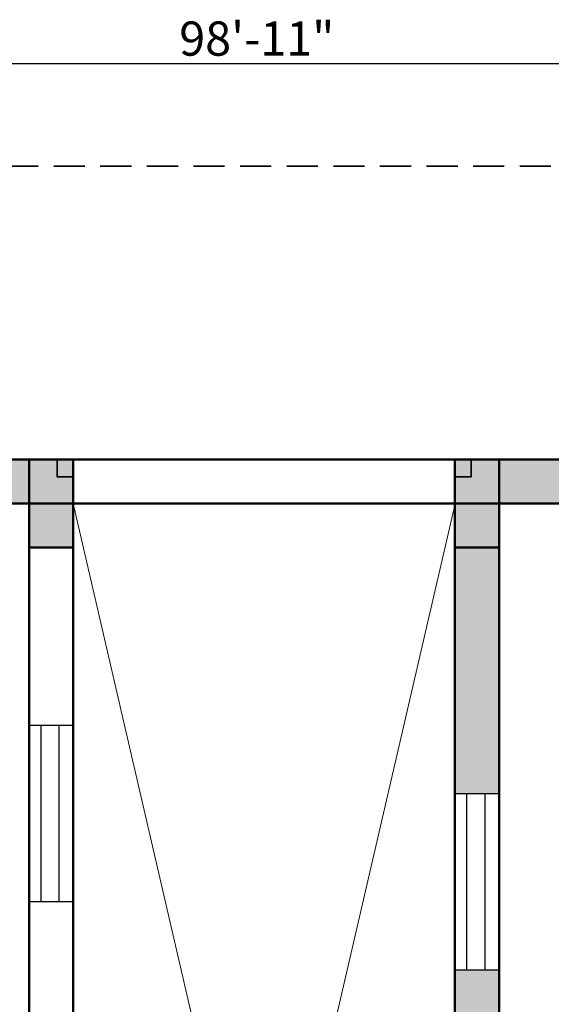
# Model space of a CAD drawing. Units: inches. Extents: x -7 to 1228, y -146 to 1091.
# Tile 77 of 88: x 545 to 654, y 890 to 1091. Entities that reach past the tile are written whole.
import ezdxf

# ---------------------------------------------------------------- set-up
doc = ezdxf.new("R2010")
doc.units = ezdxf.units.IN
doc.linetypes.add('DASHED2', pattern=[9.525, 6.35, -3.175])
for name, color, linetype, lineweight in [('A-ANNO-DIMS', 2, 'Continuous', 18), ('A-COLS', 6, 'Continuous', 35), ('A-FLOR-VOID', 7, 'Continuous', 18), ('A-GLAZ', 175, 'Continuous', 25), ('A-WALL', 7, 'Continuous', 50), ('A-WALL-PATT', 251, 'Continuous', 13), ('C-PROP', 1, 'DASHED2', 35)]:
    doc.layers.add(name, color=color, linetype=linetype, lineweight=lineweight)
doc.styles.get("Standard").update_dxf_attribs({"font": 'arial.ttf'})
doc.dimstyles.new('ISO-25', dxfattribs={"dimtxt": 7, "dimasz": 4, "dimexe": 1.25, "dimexo": 0.625, "dimtad": 1, "dimdec": 1, "dimlunit": 3, "dimtxsty": 'Standard', "dimcen": 2.5, "dimadec": 0, "dimazin": 0, "dimtfac": 1, "dimtdec": 1, "dimtmove": 1, "dimatfit": 3, "dimfxl": 1, "dimarcsym": 0})

# ---------------------------------------------------------------- blocks, each defined once
blk = doc.blocks.new('*D11')
at = {"layer": 'A-ANNO-DIMS', "color": 0, "lineweight": -2, "transparency": 16777216}
for p, q in [((0, 1061.62), (0, 1083.25)), ((4, 1082), (1183, 1082)), ((1187, 1061.62), (1187, 1083.25))]:
    blk.add_line(p, q, dxfattribs=at)
at = {"layer": 'A-ANNO-DIMS', "color": 0, "transparency": 16777216}
for points in [[(4, 1082.67), (4, 1081.33), (0, 1082)], [(1183, 1082.67), (1183, 1081.33), (1187, 1082)]]:
    blk.add_solid(points, dxfattribs=at)
at = {"layer": 'Defpoints', "color": 0, "transparency": 16777216}
for p in [(1187, 1082), (0, 1061), (1187, 1061)]:
    blk.add_point(p, dxfattribs=at)
at = {"layer": 'A-ANNO-DIMS', "color": 0, "transparency": 16777216, "insert": (593.5, 1086.2), "char_height": 7, "attachment_point": 5}
blk.add_mtext('98\'-11"', dxfattribs=at)
blk = doc.blocks.new('WIN-36')
for p, q in [((0, 36), (0, 0)), ((9, 36), (0, 36)), ((2.34, 36), (2.34, 0)), ((6.14, 0), (6.14, 36)), ((9, 0), (9, 36)), ((0, 0), (9, 0)), ((2.34, 0), (6.14, 0))]:
    blk.add_line(p, q)

msp = doc.modelspace()

# ---------------------------------------------------------------- hatches: boundary and pattern name
at = {"layer": 'A-COLS'}
h = msp.add_hatch(color=256, dxfattribs=at)
h.dxf.hatch_style = 1
h.paths.add_polyline_path([(556, 997.45), (552.71, 997.45), (552.71, 1001), (547, 1001), (547, 983), (556, 983)])
h = msp.add_hatch(color=256, dxfattribs=at)
h.dxf.hatch_style = 1
h.paths.add_polyline_path([(556, 997.45), (556, 1001), (552.71, 1001), (552.71, 997.45)])
h = msp.add_hatch(color=256, dxfattribs=at)
h.dxf.hatch_style = 1
h.paths.add_polyline_path([(634, 983), (643, 983), (643, 1001), (637.29, 1001), (637.29, 997.45), (634, 997.45)])
h = msp.add_hatch(color=256, dxfattribs=at)
h.dxf.hatch_style = 1
h.paths.add_polyline_path([(637.29, 997.45), (637.29, 1001), (634, 1001), (634, 997.45)])
at = {"layer": 'A-WALL-PATT'}
h = msp.add_hatch(color=256, dxfattribs=at)
h.dxf.hatch_style = 1
h.paths.add_polyline_path([(69, 568), (60, 568), (60, 493), (63.29, 493), (69, 493)])
h.paths.add_polyline_path([(69, 662.41), (60, 662.41), (60, 586), (69, 586)], flags=17)
h.paths.add_polyline_path([(69, 723), (184, 723), (184, 734), (179, 734), (179, 728), (69, 728), (69, 741.62), (60, 741.62), (60, 698.41), (69, 698.41)], flags=17)
h.paths.add_polyline_path([(69, 782), (231, 782), (231, 728), (231, 723), (231, 586), (236, 586), (236, 787), (69, 787), (69, 800.13), (60, 800.13), (60, 765.62), (69, 765.62)])
h.paths.add_polyline_path([(184, 842), (189, 842), (189, 848), (173, 848), (173, 842), (179, 842), (179, 787), (184, 787)])
h.paths.add_polyline_path([(118.22, 69), (69, 69), (69, 60), (118.22, 60)])
h.paths.add_polyline_path([(227, 69), (154.22, 69), (154.22, 60), (227, 60)])
h.paths.add_polyline_path([(236, 60), (232.71, 60), (227, 60), (227, 36), (236, 36)])
h.paths.add_polyline_path([(389, 60), (380, 60), (380, 36), (389, 36)])
h.paths.add_polyline_path([(384, 181), (380, 181), (380, 115), (380, 78), (384, 78)])
h.paths.add_polyline_path([(380, 115), (334.55, 115), (334.55, 109), (380, 109)])
h.paths.add_polyline_path([(274.55, 115), (236, 115), (236, 201), (232.71, 201), (231, 201), (231, 78), (236, 78), (236, 109), (274.55, 109)])
h.paths.add_polyline_path([(69, 123), (60, 123), (60, 78), (69, 78)])
h.paths.add_polyline_path([(69, 201), (60, 201), (60, 159), (69, 159)])
h.paths.add_polyline_path([(143, 219), (69, 219), (69, 213), (143, 213)], flags=17)
h.paths.add_polyline_path([(189, 219), (184, 219), (184, 274), (231, 274), (231, 219), (236, 219), (236, 279), (184, 279), (184, 297), (179, 297), (179, 279), (69, 279), (69, 290.91), (60, 290.91), (60, 262.18), (69, 262.18), (69, 274), (179, 274), (179, 219), (173, 219), (173, 213), (189, 213)])
h.paths.add_polyline_path([(69, 238.18), (60, 238.18), (60, 219), (69, 219)], flags=17)
h.paths.add_polyline_path([(69, 333), (60, 333), (60, 314.91), (69, 314.91), (69, 316.96)])
h.paths.add_polyline_path([(190, 338), (184, 338), (69, 338), (69, 333), (179, 333), (179, 327), (184, 327), (184, 333.02), (190, 333.05)])
h.paths.add_polyline_path([(69, 386.81), (60, 386.81), (60, 351), (69, 351)])
h.paths.add_polyline_path([(69, 475), (60, 475), (60, 422.81), (69, 422.81)])
h.paths.add_polyline_path([(236, 475), (231, 475), (231, 351.24), (236, 351.24)])
h.paths.add_polyline_path([(384, 475), (380, 475), (380, 362), (384, 362)])
h.paths.add_polyline_path([(547, 307), (439, 307), (439, 356), (445, 356), (445, 362), (433, 362), (433, 307), (380, 307), (380, 244), (380, 241), (384, 241), (384, 301), (433, 301), (433, 277), (439, 277), (439, 301), (547, 301)])
h.paths.add_polyline_path([(547, 241), (439, 241), (439, 247), (433, 247), (433, 235), (547, 235)])
h.paths.add_polyline_path([(450, 69), (440.29, 69), (424.89, 69), (389, 69), (389, 60), (450, 60)])
h.paths.add_polyline_path([(547, 69), (486, 69), (486, 60), (547, 60)])
h.paths.add_polyline_path([(556, 148.27), (547, 148.27), (547, 78), (556, 78)])
h.paths.add_polyline_path([(556, 223), (547, 223), (547, 195), (547, 184.27), (556, 184.27)])
h.paths.add_polyline_path([(556, 311.19), (547, 311.19), (547, 273.08), (556, 273.08)])
h.paths.add_polyline_path([(556, 344), (552.71, 344), (547, 344), (547, 335.19), (556, 335.19)])
h.paths.add_polyline_path([(556, 249.08), (547, 249.08), (547, 241), (556, 241)])
h.paths.add_polyline_path([(547, 362), (475, 362), (475, 356), (547, 356)], flags=0)
h.paths.add_polyline_path([(556, 399.62), (547, 399.62), (547, 362), (556, 362)])
h.paths.add_polyline_path([(556, 475), (547, 475), (547, 435.62), (556, 435.62)])
h.paths.add_polyline_path([(547, 493), (389, 493), (389, 487), (547, 487)])
h.paths.add_polyline_path([(380, 493), (278, 493), (278, 487), (380, 487)])
h.paths.add_polyline_path([(227, 493), (69, 493), (69, 487), (227, 487)])
h.paths.add_polyline_path([(643, 122.44), (634, 122.44), (634, 78), (643, 78)])
h.paths.add_polyline_path([(702.5, 69), (692.79, 69), (677.39, 69), (643, 69), (643, 60), (702.5, 60)])
h.paths.add_polyline_path([(798, 69), (738.5, 69), (738.5, 60), (798, 60)])
h.paths.add_polyline_path([(807, 60), (803.71, 60), (798, 60), (798, 36), (807, 36)])
h.paths.add_polyline_path([(807, 109), (846.75, 109), (846.75, 115), (807, 115), (807, 159), (802, 159), (802, 78), (807, 78)])
h.paths.add_polyline_path([(807, 201), (802, 201), (802, 195), (807, 195)])
h.paths.add_polyline_path([(643, 201), (634, 201), (634, 158.44), (643, 158.44)])
h.paths.add_polyline_path([(756, 225), (751, 225), (751, 219), (643, 219), (643, 213), (756, 213)])
h.paths.add_polyline_path([(643, 240.85), (634, 240.85), (634, 219), (643, 219)])
h.paths.add_polyline_path([(643, 274), (643, 288.63), (634, 288.63), (634, 264.85), (643, 264.85)])
h.paths.add_polyline_path([(802, 279), (756, 279), (756, 297), (751, 297), (751, 279), (643, 279), (643, 274), (751, 274), (751, 255), (756, 255), (756, 274), (802, 274)])
h.paths.add_polyline_path([(807, 333), (803.71, 333), (802, 333), (802, 279), (802, 274), (802, 219), (807, 219)])
h.paths.add_polyline_path([(956, 182), (951, 182), (951, 115), (906.75, 115), (906.75, 109), (951, 109), (951, 78), (956, 78)])
h.paths.add_polyline_path([(960, 60), (951, 60), (951, 36), (960, 36)])
h.paths.add_polyline_path([(1021, 69), (1005.78, 69), (960, 69), (960, 60), (1021, 60)])
h.paths.add_polyline_path([(956, 224), (951, 224), (951, 218), (956, 218)])
h.paths.add_polyline_path([(956, 302), (1004, 302), (1004, 278), (1010, 278), (1010, 302), (1118, 302), (1118, 290.81), (1127, 290.81), (1127, 326.97), (1118, 326.97), (1118, 320.97), (1118, 307), (1010, 307), (1010, 356), (1016, 356), (1016, 362), (1004, 362), (1004, 307), (951, 307), (951, 244), (951, 242), (954.29, 242), (956, 242)])
h.paths.add_polyline_path([(643, 333), (634, 333), (634, 312.63), (643, 312.63), (643, 316.96)])
h.paths.add_polyline_path([(756, 338), (643, 338), (643, 333), (751, 333), (751, 327), (756, 327)])
h.paths.add_polyline_path([(643, 388), (634, 388), (634, 351), (643, 351)])
h.paths.add_polyline_path([(807, 357), (802, 357), (802, 351), (807, 351)])
h.paths.add_polyline_path([(807, 475), (802, 475), (802, 393), (807, 393)])
h.paths.add_polyline_path([(643, 475), (634, 475), (634, 424), (643, 424)])
h.paths.add_polyline_path([(798, 493), (643, 493), (643, 487), (798, 487)])
h.paths.add_polyline_path([(634, 493), (556, 493), (556, 487), (634, 487)])
h.paths.add_polyline_path([(813, 493), (807, 493), (807, 487), (813, 487)])
h.paths.add_polyline_path([(951, 493), (849, 493), (849, 487), (951, 487)])
h.paths.add_polyline_path([(956, 484), (951, 484), (951, 374), (956, 374)])
h.paths.add_polyline_path([(1109, 493), (969, 493), (969, 487), (1109, 487)])
h.paths.add_polyline_path([(1127, 484), (1118, 484), (1118, 450.64), (1127, 450.64)])
h.paths.add_polyline_path([(1127, 414.64), (1118, 414.64), (1118, 365), (1127, 365)])
h.paths.add_polyline_path([(1109, 362), (1046, 362), (1046, 356), (1109, 356)], flags=17)
h.paths.add_polyline_path([(1127, 356), (1123.45, 356), (1118, 356), (1118, 350.97), (1127, 350.97)], flags=0)
h.paths.add_polyline_path([(1127, 266.81), (1118, 266.81), (1118, 262.36), (1118, 242), (1127, 242)], flags=17)
h.paths.add_polyline_path([(1118, 242), (1010, 242), (1010, 248), (1004, 248), (1004, 237), (1118, 237)])
h.paths.add_polyline_path([(1127, 224), (1118, 224), (1118, 170), (1127, 170)])
h.paths.add_polyline_path([(1127, 134), (1118, 134), (1118, 78), (1127, 78)])
h.paths.add_polyline_path([(1118, 69), (1057, 69), (1057, 60), (1118, 60)])
h.paths.add_polyline_path([(227, 571.55), (227, 574), (69, 574), (69, 568), (227, 568)])
h.paths.add_polyline_path([(380, 571.55), (380, 574), (278, 574), (278, 568), (380, 568)])
h.paths.add_polyline_path([(242, 574), (236, 574), (236, 568), (242, 568)])
h.paths.add_polyline_path([(547, 571.55), (547, 574), (389, 574), (389, 568), (547, 568)])
h.paths.add_polyline_path([(384, 733), (380, 733), (380, 586), (384, 586)])
h.paths.add_polyline_path([(556, 646), (634, 646), (634, 655), (547, 655), (547, 586), (556, 586)])
h.paths.add_polyline_path([(634, 574), (556, 574), (556, 568), (634, 568)])
h.paths.add_polyline_path([(643, 655), (634, 655), (634, 586), (643, 586)])
h.paths.add_polyline_path([(798, 574), (643, 574), (643, 568), (798, 568)])
h.paths.add_polyline_path([(643, 663.85), (634, 663.85), (634, 655), (643, 655)])
h.paths.add_polyline_path([(556, 676.97), (547, 676.97), (547, 655), (556, 655)])
h.paths.add_polyline_path([(556, 733), (547, 733), (547, 712.97), (556, 712.97)])
h.paths.add_polyline_path([(643, 710), (634, 710), (634, 699.85), (643, 699.85)])
h.paths.add_polyline_path([(807, 668), (802, 668), (802, 586), (807, 586)])
h.paths.add_polyline_path([(951, 574), (849, 574), (849, 568), (951, 568)])
h.paths.add_polyline_path([(956, 691), (951, 691), (951, 577), (956, 577)])
h.paths.add_polyline_path([(1109, 574), (969, 574), (969, 568), (1109, 568)])
h.paths.add_polyline_path([(1127, 643.4), (1118, 643.4), (1118, 577), (1127, 577)])
h.paths.add_polyline_path([(1127, 568), (1123.45, 568), (1118, 568), (1118, 493), (1127, 493)])
h.paths.add_polyline_path([(1127, 733), (1118, 733), (1118, 679.4), (1127, 679.4)])
h.paths.add_polyline_path([(1127, 777.35), (1118, 777.35), (1118, 770.04), (1118, 751), (1127, 751)], flags=17)
h.paths.add_polyline_path([(1118, 751), (1010, 751), (1010, 757), (1004, 757), (1004, 745), (1118, 745)])
h.paths.add_polyline_path([(956, 811), (1004, 811), (1004, 787), (1010, 787), (1010, 811), (1017.87, 811), (1017.87, 811.63, -0.414214), (1018.25, 812), (1031.98, 812, -0.414214), (1032.35, 811.63), (1032.35, 811), (1118, 811), (1118, 801.35), (1127, 801.35), (1127, 834.69), (1118, 834.69), (1118, 830.24), (1118, 817), (1010, 817), (1010, 866), (1016, 866), (1016, 872), (1004, 872), (1004, 817), (956, 817), (956, 866), (951, 866), (951, 751), (954.29, 751), (956, 751)])
h.paths.add_polyline_path([(1118, 872), (1046, 872), (1046, 866), (1118, 866)], flags=17)
h.paths.add_polyline_path([(1127, 924.71), (1118, 924.71), (1118, 884), (1127, 884)])
h.paths.add_polyline_path([(1127, 866), (1123.71, 866), (1118, 866), (1118, 858.69), (1127, 858.69)], flags=17)
h.paths.add_polyline_path([(956, 983), (951, 983), (951, 952), (807, 952), (807, 983), (802, 983), (802, 902), (807, 902), (807, 946), (951, 946), (951, 884), (956, 884)])
h.paths.add_polyline_path([(807, 842), (802, 842), (802, 787), (756, 787), (756, 806), (751, 806), (751, 787), (643, 787), (643, 782), (751, 782), (751, 764), (756, 764), (756, 782), (802, 782), (802, 728), (807, 728)])
h.paths.add_polyline_path([(756, 848), (643, 848), (643, 842), (751, 842), (751, 836), (756, 836)])
h.paths.add_polyline_path([(756, 734), (751, 734), (751, 728), (643, 728), (643, 723), (756, 723)])
h.paths.add_polyline_path([(643, 749.79), (634, 749.79), (634, 728), (637.29, 728), (643, 728)])
h.paths.add_polyline_path([(643, 805.41), (634, 805.41), (634, 773.79), (643, 773.79)])
h.paths.add_polyline_path([(643, 896.66), (634, 896.66), (634, 860), (637.29, 860), (643, 860)])
h.paths.add_polyline_path([(643, 842), (634, 842), (634, 829.41), (643, 829.41)])
h.paths.add_polyline_path([(643, 983), (634, 983), (634, 932.66), (643, 932.66)])
h.paths.add_polyline_path([(1127, 983), (1118, 983), (1118, 960.71), (1127, 960.71)])
h.paths.add_polyline_path([(1118, 1001), (1077.53, 1001), (1077.53, 992), (1118, 992)])
h.paths.add_polyline_path([(1041.53, 1001), (960, 1001), (960, 992), (1041.53, 992)])
h.paths.add_polyline_path([(960, 1025), (951, 1025), (951, 1001), (954.29, 1001), (960, 1001)])
h.paths.add_polyline_path([(807, 1025), (798, 1025), (798, 1001), (807, 1001)])
h.paths.add_polyline_path([(798, 1001), (738.5, 1001), (738.5, 992), (798, 992)])
h.paths.add_polyline_path([(702.5, 1001), (643, 1001), (643, 992), (702.5, 992)])
h.paths.add_polyline_path([(547, 1001), (499.11, 1001), (499.11, 992), (547, 992)])
h.paths.add_polyline_path([(463.11, 1001), (389, 1001), (389, 992), (463.11, 992)])
h.paths.add_polyline_path([(389, 1025), (380, 1025), (380, 1022), (380, 1001), (383.29, 1001), (389, 1001)])
h.paths.add_polyline_path([(236, 1025), (227, 1025), (227, 1001), (236, 1001)])
h.paths.add_polyline_path([(236, 983), (231, 983), (231, 860), (236, 860)])
h.paths.add_polyline_path([(274.55, 952), (236, 952), (236, 946), (274.55, 946)])
h.paths.add_polyline_path([(380, 952), (334.55, 952), (334.55, 946), (380, 946)])
h.paths.add_polyline_path([(384, 983), (380, 983), (380, 884), (383.29, 884), (384, 884)])
h.paths.add_polyline_path([(227, 1001), (155.01, 1001), (155.01, 992), (162.87, 992), (227, 992)])
h.paths.add_polyline_path([(119.01, 1001), (69, 1001), (69, 992), (119.01, 992)])
h.paths.add_polyline_path([(69, 983), (60, 983), (60, 922.99), (69, 922.99)])
h.paths.add_polyline_path([(69, 886.99), (60, 886.99), (60, 860), (63.29, 860), (69, 860)])
h.paths.add_polyline_path([(143, 848), (69, 848), (69, 842), (143, 842)])

# ---------------------------------------------------------------- linework, layer by layer
at = {"layer": 'A-COLS'}
for points in [[(556, 1001), (552.71, 1001), (552.71, 997.45), (556, 997.45)], [(634, 1001), (637.29, 1001), (637.29, 997.45), (634, 997.45)]]:
    msp.add_lwpolyline(points, close=True, dxfattribs=at)
at = {"layer": 'A-FLOR-VOID'}
for p, q in [((556, 992), (634, 655)), ((556, 655), (634, 991.66))]:
    msp.add_line(p, q, dxfattribs=at)
at = {"layer": 'A-WALL'}
for p, q in [((556, 1001), (380, 1001)), ((547, 1001), (547, 872)), ((556, 1001), (547, 1001)), ((547, 1001), (547, 983)), ((556, 1001), (556, 655)), ((556, 992), (556, 1001)), ((556, 1001), (556, 1001)), ((556, 983), (556, 1001)), ((634, 1001), (556, 1001)), ((634, 1001), (634, 655)), ((634, 1001), (643, 1001)), ((634, 983), (634, 1001)), ((807, 1001), (634, 1001)), ((634, 568), (634, 1001)), ((643, 1001), (643, 848)), ((643, 1001), (643, 983)), ((643, 568), (643, 1001)), ((556, 992), (380, 992)), ((634, 992), (556, 992)), ((807, 992), (634, 992)), ((547, 983), (556, 983)), ((643, 983), (634, 983))]:
    msp.add_line(p, q, dxfattribs=at)
at = {"layer": 'C-PROP'}
msp.add_line((1187, 1061), (0, 1061), dxfattribs=at)

# ---------------------------------------------------------------- block references
at = {"layer": 'A-GLAZ'}
for p in [(547, 910.65), (634, 896.66)]:
    msp.add_blockref('WIN-36', p, dxfattribs=at)

# ---------------------------------------------------------------- dimensions: what is measured, and where the dimension line sits
at = {"layer": 'A-ANNO-DIMS'}
dim = msp.add_linear_dim(base=(1187, 1082), p1=(0, 1061), p2=(1187, 1061), dimstyle='ISO-25', override={"dimclrd": 0, "dimclre": 0, "dimclrt": 0}, dxfattribs=at)
dim.commit()
dim.dimension.update_dxf_attribs({"geometry": '*D11', "text_midpoint": (593.5, 1086.2)})

doc.saveas('drawing.dxf')
